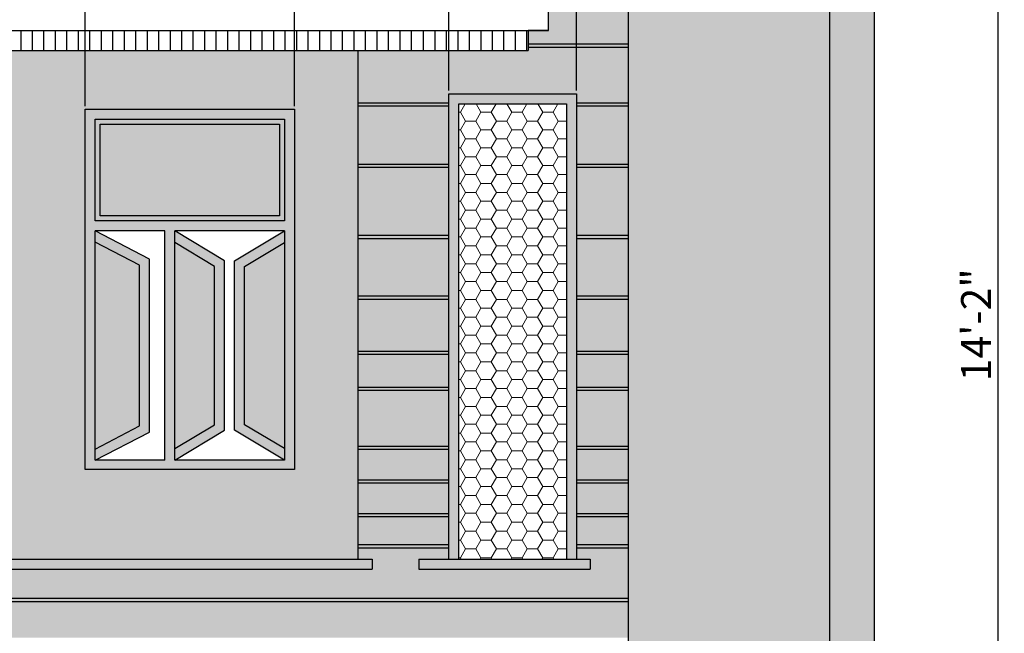
# Model space of a CAD drawing. Units: millimetres. Extents: x 4237 to 5109, y 21391 to 22486.
# Tile 3 of 17: x 4911 to 5109, y 21581 to 21704. Entities that reach past the tile are written whole.
import ezdxf

# ---------------------------------------------------------------- set-up
doc = ezdxf.new("R2010")
doc.units = ezdxf.units.MM
for name, color, linetype, lineweight in [('A-ANNO-DIMS', 2, 'Continuous', 18), ('A-ELEV', 7, 'Continuous', 25), ('A-ELEV-PATT', 252, 'Continuous', 13)]:
    doc.layers.add(name, color=color, linetype=linetype, lineweight=lineweight)
doc.styles.get("Standard").update_dxf_attribs({"font": 'arial.ttf'})
doc.dimstyles.new('ISO-25', dxfattribs={"dimtxt": 6, "dimasz": 2.5, "dimexe": 1.25, "dimexo": 0.625, "dimtad": 1, "dimdec": 1, "dimlunit": 4, "dimtxsty": 'Standard', "dimcen": 2.5, "dimadec": 0, "dimazin": 0, "dimtfac": 1, "dimtdec": 1, "dimtmove": 0, "dimatfit": 3, "dimfxl": 1, "dimarcsym": 0})

# ---------------------------------------------------------------- blocks, each defined once
blk = doc.blocks.new('*D130')
at = {"layer": 'A-ANNO-DIMS', "color": 0, "lineweight": -2, "transparency": 16777216}
for p, q in [((4878.54, 21688.54), (4878.54, 21897.84)), ((4881.04, 21896.59), (4921.78, 21896.59)), ((4924.28, 21686.68), (4924.28, 21897.84))]:
    blk.add_line(p, q, dxfattribs=at)
at = {"layer": 'A-ANNO-DIMS', "color": 0, "transparency": 16777216}
for points in [[(4881.04, 21897), (4881.04, 21896.17), (4878.54, 21896.59)], [(4921.78, 21897), (4921.78, 21896.17), (4924.28, 21896.59)]]:
    blk.add_solid(points, dxfattribs=at)
at = {"layer": 'Defpoints', "color": 0, "transparency": 16777216}
for p in [(4924.28, 21896.59), (4878.54, 21687.91), (4924.28, 21686.05)]:
    blk.add_point(p, dxfattribs=at)
at = {"layer": 'A-ANNO-DIMS', "color": 0, "transparency": 16777216, "insert": (4901.41, 21900.32), "char_height": 6, "attachment_point": 5}
blk.add_mtext('3\'-9 1/2"', dxfattribs=at)
blk = doc.blocks.new('*D131')
at = {"layer": 'A-ANNO-DIMS', "color": 0, "lineweight": -2, "transparency": 16777216}
for p, q in [((4924.28, 21686.68), (4924.28, 21897.84)), ((4926.78, 21896.59), (4963.73, 21896.59)), ((4966.23, 21686.68), (4966.23, 21897.84))]:
    blk.add_line(p, q, dxfattribs=at)
at = {"layer": 'A-ANNO-DIMS', "color": 0, "transparency": 16777216}
for points in [[(4926.78, 21897), (4926.78, 21896.17), (4924.28, 21896.59)], [(4963.73, 21897), (4963.73, 21896.17), (4966.23, 21896.59)]]:
    blk.add_solid(points, dxfattribs=at)
at = {"layer": 'Defpoints', "color": 0, "transparency": 16777216}
for p in [(4966.23, 21896.59), (4924.28, 21686.05), (4966.23, 21686.05)]:
    blk.add_point(p, dxfattribs=at)
at = {"layer": 'A-ANNO-DIMS', "color": 0, "transparency": 16777216, "insert": (4945.25, 21900.28), "char_height": 6, "attachment_point": 5}
blk.add_mtext('3\'-6"', dxfattribs=at)
blk = doc.blocks.new('*D132')
at = {"layer": 'A-ANNO-DIMS', "color": 0, "lineweight": -2, "transparency": 16777216}
for p, q in [((4966.23, 21686.68), (4966.23, 21897.84)), ((4968.73, 21896.59), (4994.7, 21896.59)), ((4997.2, 21689.78), (4997.2, 21897.84))]:
    blk.add_line(p, q, dxfattribs=at)
at = {"layer": 'A-ANNO-DIMS', "color": 0, "transparency": 16777216}
for points in [[(4968.73, 21897), (4968.73, 21896.17), (4966.23, 21896.59)], [(4994.7, 21897), (4994.7, 21896.17), (4997.2, 21896.59)]]:
    blk.add_solid(points, dxfattribs=at)
at = {"layer": 'Defpoints', "color": 0, "transparency": 16777216}
for p in [(4997.2, 21896.59), (4997.2, 21689.16), (4966.23, 21686.05)]:
    blk.add_point(p, dxfattribs=at)
at = {"layer": 'A-ANNO-DIMS', "color": 0, "transparency": 16777216, "insert": (4981.72, 21900.22), "char_height": 6, "attachment_point": 5}
blk.add_mtext('2\'-7"', dxfattribs=at)
blk = doc.blocks.new('*D133')
at = {"layer": 'A-ANNO-DIMS', "color": 0, "lineweight": -2, "transparency": 16777216}
for p, q in [((4997.2, 21689.78), (4997.2, 21897.84)), ((4999.7, 21896.59), (5020.26, 21896.59)), ((5022.76, 21689.78), (5022.76, 21897.84)), ((5022.76, 21896.59), (5056.55, 21896.59))]:
    blk.add_line(p, q, dxfattribs=at)
at = {"layer": 'A-ANNO-DIMS', "color": 0, "transparency": 16777216}
for points in [[(4999.7, 21897), (4999.7, 21896.17), (4997.2, 21896.59)], [(5020.26, 21897), (5020.26, 21896.17), (5022.76, 21896.59)]]:
    blk.add_solid(points, dxfattribs=at)
at = {"layer": 'Defpoints', "color": 0, "transparency": 16777216}
for p in [(5022.76, 21896.59), (4997.2, 21689.16), (5022.76, 21689.16)]:
    blk.add_point(p, dxfattribs=at)
at = {"layer": 'A-ANNO-DIMS', "color": 0, "transparency": 16777216, "insert": (5040.91, 21900.31), "char_height": 6, "attachment_point": 5}
blk.add_mtext('2\'-1 1/2"', dxfattribs=at)
blk = doc.blocks.new('*D134')
at = {"layer": 'A-ANNO-DIMS', "color": 0, "lineweight": -2, "transparency": 16777216}
for p, q in [((5022.76, 21689.78), (5022.76, 21897.84)), ((5025.26, 21896.59), (5080.03, 21896.59)), ((5082.53, 21809.46), (5082.53, 21897.84))]:
    blk.add_line(p, q, dxfattribs=at)
at = {"layer": 'A-ANNO-DIMS', "color": 0, "transparency": 16777216}
for points in [[(5025.26, 21897), (5025.26, 21896.17), (5022.76, 21896.59)], [(5080.03, 21897), (5080.03, 21896.17), (5082.53, 21896.59)]]:
    blk.add_solid(points, dxfattribs=at)
at = {"layer": 'Defpoints', "color": 0, "transparency": 16777216}
for p in [(5082.53, 21896.59), (5082.53, 21808.84), (5022.76, 21689.16)]:
    blk.add_point(p, dxfattribs=at)
at = {"layer": 'A-ANNO-DIMS', "color": 0, "transparency": 16777216, "insert": (5052.65, 21900.27), "char_height": 6, "attachment_point": 5}
blk.add_mtext('5\'-0"', dxfattribs=at)
blk = doc.blocks.new('*D136')
at = {"layer": 'A-ANNO-DIMS', "color": 0, "lineweight": -2, "transparency": 16777216}
for p, q in [((5074.15, 21727.84), (5108.53, 21727.84)), ((5107.28, 21560.34), (5107.28, 21725.34)), ((5083.15, 21557.84), (5108.53, 21557.84))]:
    blk.add_line(p, q, dxfattribs=at)
at = {"layer": 'A-ANNO-DIMS', "color": 0, "transparency": 16777216}
for points in [[(5106.86, 21725.34), (5107.69, 21725.34), (5107.28, 21727.84)], [(5106.86, 21560.34), (5107.69, 21560.34), (5107.28, 21557.84)]]:
    blk.add_solid(points, dxfattribs=at)
at = {"layer": 'Defpoints', "color": 0, "transparency": 16777216}
for p in [(5073.53, 21727.84), (5107.28, 21727.84), (5082.53, 21557.84)]:
    blk.add_point(p, dxfattribs=at)
at = {"layer": 'A-ANNO-DIMS', "color": 0, "transparency": 16777216, "insert": (5103.64, 21642.84), "char_height": 6, "attachment_point": 5, "rotation": 90}
blk.add_mtext('14\'-2"', dxfattribs=at)

msp = doc.modelspace()

# ---------------------------------------------------------------- hatches: boundary and pattern name
at = {"layer": 'A-ELEV-PATT'}
h = msp.add_hatch(color=256, dxfattribs=at)
h.dxf.hatch_style = 1
h.paths.add_polyline_path([(4957.45, 21796.84), (4963.45, 21796.84), (4963.45, 21727.84), (4966.45, 21727.84), (4966.45, 21796.84), (4972.45, 21796.84), (4972.45, 21727.84), (4975.45, 21727.84), (4975.45, 21796.84), (4981.45, 21796.84), (4981.45, 21727.84), (4984.45, 21727.84), (4984.45, 21796.84), (5073.53, 21796.84), (5073.53, 21557.84), (5082.53, 21557.84), (5082.53, 21808.84), (4951.45, 21808.84), (4951.45, 21727.84), (4957.45, 21727.84)])
h = msp.add_hatch(color=256, dxfattribs=at)
h.dxf.hatch_style = 1
h.paths.add_polyline_path([(5073.53, 21725.84), (5033.17, 21725.84), (5033.17, 21557.84), (5073.53, 21557.84)])
h = msp.add_hatch(color=256, dxfattribs=at)
h.dxf.hatch_style = 1
h.paths.add_polyline_path([(5033.17, 21707.76), (5017.14, 21707.76), (5017.14, 21701.84), (5013.1, 21701.84), (5013.1, 21699.14), (5033.17, 21699.14)])
h = msp.add_hatch(color=256, dxfattribs=at)
h.dxf.hatch_style = 1
h.paths.add_polyline_path([(5033.17, 21699.14), (5013.1, 21699.14), (5013.1, 21698.51), (5033.17, 21698.51)])
h = msp.add_hatch(color=256, dxfattribs=at)
h.dxf.hatch_style = 1
h.paths.add_polyline_path([(4978.93, 21697.84), (4892.07, 21697.84), (4892.07, 21623.26), (4900.89, 21623.26, -1), (4900.89, 21620.26), (4892.07, 21620.26), (4892.07, 21615.26), (4900.89, 21615.26, -1), (4900.89, 21613.26), (4892.07, 21613.26), (4892.07, 21608.26), (4900.89, 21608.26, -1), (4900.89, 21606.26), (4892.07, 21606.26), (4892.07, 21601.26), (4900.89, 21601.26, -1), (4900.89, 21599.26), (4892.07, 21599.26), (4892.07, 21595.84), (4978.93, 21595.84)])
h.paths.add_polyline_path([(4924.28, 21686.05), (4966.23, 21686.05), (4966.23, 21613.83), (4924.28, 21613.83)], flags=16)
h.paths.add_polyline_path([(4926.28, 21661.68), (4940.28, 21661.68), (4940.28, 21615.68), (4926.28, 21615.68)], flags=0)
h.paths.add_polyline_path([(4942.28, 21661.68), (4964.23, 21661.68), (4964.23, 21615.68), (4942.28, 21615.68)], flags=0)
h.paths.add_polyline_path([(4926.28, 21663.68), (4926.28, 21684.05), (4964.23, 21684.05), (4964.23, 21663.68)], flags=0)
h.paths.add_polyline_path([(4927.28, 21664.68), (4927.28, 21683.05), (4963.23, 21683.05), (4963.23, 21664.68)], flags=0)
h = msp.add_hatch(color=256, dxfattribs=at)
h.dxf.hatch_style = 1
h.paths.add_polyline_path([(5033.17, 21698.51), (5013.1, 21698.51), (5013.1, 21697.84), (4978.93, 21697.84), (4978.93, 21687.37), (4997.2, 21687.37), (4997.2, 21689.16), (5022.76, 21689.16), (5022.76, 21687.37), (5033.17, 21687.37)])
h = msp.add_hatch(color=256, dxfattribs=at)
h.dxf.hatch_style = 1
h.paths.add_polyline_path([(5022.76, 21689.16), (4997.2, 21689.16), (4997.2, 21595.84), (4999.2, 21595.84), (4999.2, 21687.16), (5020.76, 21687.16), (5020.76, 21595.84), (5022.76, 21595.84)])
h = msp.add_hatch(color=256, dxfattribs=at)
h.dxf.hatch_style = 1
h.paths.add_polyline_path([(4997.2, 21687.37), (4978.93, 21687.37), (4978.93, 21686.74), (4997.2, 21686.74)])
h = msp.add_hatch(dxfattribs=at)
h.set_pattern_fill('HONEY', color=256, scale=0.65)
h.set_pattern_definition([(0, (437.5752, 168.6426), (3.095625, 1.78725992), [2.06375, -4.1275]), (120, (437.5752, 168.6426), (-3.095625, 1.78725993), [2.06375, -4.1275]), (60, (437.5752, 168.6426), (7e-09, 3.57451985), [-4.1275, 2.06375])])
h.paths.add_polyline_path([(5020.76, 21687.16), (4999.2, 21687.16), (4999.2, 21595.84), (5020.76, 21595.84)])
h = msp.add_hatch(color=256, dxfattribs=at)
h.dxf.hatch_style = 1
h.paths.add_polyline_path([(5033.17, 21687.37), (5022.76, 21687.37), (5022.76, 21686.74), (5033.17, 21686.74)])
h = msp.add_hatch(color=256, dxfattribs=at)
h.dxf.hatch_style = 1
h.paths.add_polyline_path([(4966.23, 21686.05), (4924.28, 21686.05), (4924.28, 21613.83), (4966.23, 21613.83)])
h.paths.add_polyline_path([(4964.23, 21615.68), (4942.28, 21615.68), (4942.28, 21661.68), (4964.23, 21661.68)], flags=16)
h.paths.add_polyline_path([(4964.23, 21663.68), (4926.28, 21663.68), (4926.28, 21684.05), (4964.23, 21684.05)], flags=16)
h.paths.add_polyline_path([(4963.23, 21664.68), (4927.28, 21664.68), (4927.28, 21683.05), (4963.23, 21683.05)], flags=0)
h.paths.add_polyline_path([(4940.28, 21615.68), (4926.28, 21615.68), (4926.28, 21661.68), (4940.28, 21661.68)], flags=16)
h = msp.add_hatch(color=256, dxfattribs=at)
h.dxf.hatch_style = 1
h.paths.add_polyline_path([(4997.2, 21686.74), (4978.93, 21686.74), (4978.93, 21675.04), (4997.2, 21675.04)])
h = msp.add_hatch(color=256, dxfattribs=at)
h.dxf.hatch_style = 1
h.paths.add_polyline_path([(5033.17, 21686.74), (5022.76, 21686.74), (5022.76, 21675.04), (5033.17, 21675.04)])
h = msp.add_hatch(color=256, dxfattribs=at)
h.dxf.hatch_style = 1
h.set_gradient(color1=(122, 175, 223), color2=(215, 235, 210), name='CYLINDER')
h.paths.add_polyline_path([(4964.23, 21684.05), (4926.28, 21684.05), (4926.28, 21663.68), (4964.23, 21663.68)])
h.paths.add_polyline_path([(4963.23, 21683.05), (4963.23, 21664.68), (4927.28, 21664.68), (4927.28, 21683.05)], flags=16)
h = msp.add_hatch(color=256, dxfattribs=at)
h.dxf.hatch_style = 1
h.set_gradient(color1=(122, 175, 223), color2=(215, 235, 210), name='HEMISPHERICAL')
h.paths.add_polyline_path([(4963.23, 21683.05), (4927.28, 21683.05), (4927.28, 21664.68), (4963.23, 21664.68)])
h = msp.add_hatch(color=256, dxfattribs=at)
h.dxf.hatch_style = 1
h.paths.add_polyline_path([(4997.2, 21675.04), (4978.93, 21675.04), (4978.93, 21674.41), (4997.2, 21674.41)])
h = msp.add_hatch(color=256, dxfattribs=at)
h.dxf.hatch_style = 1
h.paths.add_polyline_path([(4997.2, 21674.41), (4978.93, 21674.41), (4978.93, 21660.8), (4997.2, 21660.8)])
h = msp.add_hatch(color=256, dxfattribs=at)
h.dxf.hatch_style = 1
h.paths.add_polyline_path([(5033.17, 21675.04), (5022.76, 21675.04), (5022.76, 21674.41), (5033.17, 21674.41)])
h = msp.add_hatch(color=256, dxfattribs=at)
h.dxf.hatch_style = 1
h.paths.add_polyline_path([(5033.17, 21674.41), (5022.76, 21674.41), (5022.76, 21660.8), (5033.17, 21660.8)])
h = msp.add_hatch(color=256, dxfattribs=at)
h.dxf.hatch_style = 1
h.paths.add_polyline_path([(4937.18, 21656.02), (4926.28, 21661.68), (4926.28, 21659.42), (4935.18, 21654.81), (4935.18, 21622.55), (4926.28, 21617.93), (4926.28, 21615.68), (4937.18, 21621.33)])
h = msp.add_hatch(color=256, dxfattribs=at)
h.dxf.hatch_style = 1
h.paths.add_polyline_path([(4952.25, 21655.67), (4942.28, 21661.68), (4942.28, 21659.34), (4950.25, 21654.54), (4950.25, 21622.81), (4942.28, 21618.01), (4942.28, 21615.68), (4952.25, 21621.68)])
h = msp.add_hatch(color=256, dxfattribs=at)
h.dxf.hatch_style = 1
h.paths.add_polyline_path([(4956.25, 21654.54), (4964.23, 21659.34), (4964.23, 21661.68), (4954.25, 21655.67), (4954.25, 21621.68), (4964.23, 21615.68), (4964.23, 21618.01), (4956.25, 21622.81)])
h = msp.add_hatch(color=256, dxfattribs=at)
h.dxf.hatch_style = 1
h.set_gradient(color1=(122, 175, 223), color2=(215, 235, 210), name='INVCYLINDER')
h.paths.add_polyline_path([(4935.18, 21654.81), (4926.28, 21659.42), (4926.28, 21617.93), (4935.18, 21622.55)])
h = msp.add_hatch(color=256, dxfattribs=at)
h.dxf.hatch_style = 1
h.paths.add_polyline_path([(4997.2, 21660.8), (4978.93, 21660.8), (4978.93, 21660.17), (4997.2, 21660.17)])
h = msp.add_hatch(color=256, dxfattribs=at)
h.dxf.hatch_style = 1
h.paths.add_polyline_path([(4997.2, 21660.17), (4978.93, 21660.17), (4978.93, 21648.61), (4997.2, 21648.61)])
h = msp.add_hatch(color=256, dxfattribs=at)
h.dxf.hatch_style = 1
h.paths.add_polyline_path([(5033.17, 21660.8), (5022.76, 21660.8), (5022.76, 21660.17), (5033.17, 21660.17)])
h = msp.add_hatch(color=256, dxfattribs=at)
h.dxf.hatch_style = 1
h.paths.add_polyline_path([(5033.17, 21660.17), (5022.76, 21660.17), (5022.76, 21648.61), (5033.17, 21648.61)])
h = msp.add_hatch(color=256, dxfattribs=at)
h.dxf.hatch_style = 1
h.set_gradient(color1=(122, 175, 223), color2=(215, 235, 210), name='INVCYLINDER')
h.paths.add_polyline_path([(4950.25, 21654.54), (4942.28, 21659.34), (4942.28, 21618.01), (4950.25, 21622.81)])
h = msp.add_hatch(color=256, dxfattribs=at)
h.dxf.hatch_style = 1
h.set_gradient(color1=(122, 175, 223), color2=(215, 235, 210), name='INVCYLINDER')
h.paths.add_polyline_path([(4964.23, 21659.34), (4956.25, 21654.54), (4956.25, 21622.81), (4964.23, 21618.01)])
h = msp.add_hatch(color=256, dxfattribs=at)
h.dxf.hatch_style = 1
h.paths.add_polyline_path([(4997.2, 21648.61), (4978.93, 21648.61), (4978.93, 21647.98), (4997.2, 21647.98)])
h = msp.add_hatch(color=256, dxfattribs=at)
h.dxf.hatch_style = 1
h.paths.add_polyline_path([(4997.2, 21647.98), (4978.93, 21647.98), (4978.93, 21637.57), (4997.2, 21637.57)])
h = msp.add_hatch(color=256, dxfattribs=at)
h.dxf.hatch_style = 1
h.paths.add_polyline_path([(5033.17, 21648.61), (5022.76, 21648.61), (5022.76, 21647.98), (5033.17, 21647.98)])
h = msp.add_hatch(color=256, dxfattribs=at)
h.dxf.hatch_style = 1
h.paths.add_polyline_path([(5033.17, 21647.98), (5022.76, 21647.98), (5022.76, 21637.57), (5033.17, 21637.57)])
h = msp.add_hatch(color=256, dxfattribs=at)
h.dxf.hatch_style = 1
h.paths.add_polyline_path([(4997.2, 21637.57), (4978.93, 21637.57), (4978.93, 21636.94), (4997.2, 21636.94)])
h = msp.add_hatch(color=256, dxfattribs=at)
h.dxf.hatch_style = 1
h.paths.add_polyline_path([(4997.2, 21636.94), (4978.93, 21636.94), (4978.93, 21630.34), (4997.2, 21630.34)])
h = msp.add_hatch(color=256, dxfattribs=at)
h.dxf.hatch_style = 1
h.paths.add_polyline_path([(5033.17, 21637.57), (5022.76, 21637.57), (5022.76, 21636.94), (5033.17, 21636.94)])
h = msp.add_hatch(color=256, dxfattribs=at)
h.dxf.hatch_style = 1
h.paths.add_polyline_path([(5033.17, 21636.94), (5022.76, 21636.94), (5022.76, 21630.34), (5033.17, 21630.34)])
h = msp.add_hatch(color=256, dxfattribs=at)
h.dxf.hatch_style = 1
h.paths.add_polyline_path([(4997.2, 21630.34), (4978.93, 21630.34), (4978.93, 21629.72), (4997.2, 21629.72)])
h = msp.add_hatch(color=256, dxfattribs=at)
h.dxf.hatch_style = 1
h.paths.add_polyline_path([(5033.17, 21630.34), (5022.76, 21630.34), (5022.76, 21629.72), (5033.17, 21629.72)])
h = msp.add_hatch(color=256, dxfattribs=at)
h.dxf.hatch_style = 1
h.paths.add_polyline_path([(4997.2, 21629.72), (4978.93, 21629.72), (4978.93, 21618.5), (4997.2, 21618.5)])
h = msp.add_hatch(color=256, dxfattribs=at)
h.dxf.hatch_style = 1
h.paths.add_polyline_path([(5033.17, 21629.72), (5022.76, 21629.72), (5022.76, 21618.5), (5033.17, 21618.5)])
h = msp.add_hatch(color=256, dxfattribs=at)
h.dxf.hatch_style = 1
h.paths.add_polyline_path([(4997.2, 21618.5), (4978.93, 21618.5), (4978.93, 21617.88), (4997.2, 21617.88)])
h = msp.add_hatch(color=256, dxfattribs=at)
h.dxf.hatch_style = 1
h.paths.add_polyline_path([(5033.17, 21618.5), (5022.76, 21618.5), (5022.76, 21617.88), (5033.17, 21617.88)])
h = msp.add_hatch(color=256, dxfattribs=at)
h.dxf.hatch_style = 1
h.paths.add_polyline_path([(4997.2, 21617.88), (4978.93, 21617.88), (4978.93, 21611.76), (4997.2, 21611.76)])
h = msp.add_hatch(color=256, dxfattribs=at)
h.dxf.hatch_style = 1
h.paths.add_polyline_path([(5033.17, 21617.88), (5022.76, 21617.88), (5022.76, 21611.76), (5033.17, 21611.76)])
h = msp.add_hatch(color=256, dxfattribs=at)
h.dxf.hatch_style = 1
h.paths.add_polyline_path([(4997.2, 21611.76), (4978.93, 21611.76), (4978.93, 21611.13), (4997.2, 21611.13)])
h = msp.add_hatch(color=256, dxfattribs=at)
h.dxf.hatch_style = 1
h.paths.add_polyline_path([(4997.2, 21611.13), (4978.93, 21611.13), (4978.93, 21605.02), (4997.2, 21605.02)])
h = msp.add_hatch(color=256, dxfattribs=at)
h.dxf.hatch_style = 1
h.paths.add_polyline_path([(5033.17, 21611.76), (5022.76, 21611.76), (5022.76, 21611.13), (5033.17, 21611.13)])
h = msp.add_hatch(color=256, dxfattribs=at)
h.dxf.hatch_style = 1
h.paths.add_polyline_path([(5033.17, 21611.13), (5022.76, 21611.13), (5022.76, 21605.02), (5033.17, 21605.02)])
h = msp.add_hatch(color=256, dxfattribs=at)
h.dxf.hatch_style = 1
h.paths.add_polyline_path([(4997.2, 21605.02), (4978.93, 21605.02), (4978.93, 21604.39), (4997.2, 21604.39)])
h = msp.add_hatch(color=256, dxfattribs=at)
h.dxf.hatch_style = 1
h.paths.add_polyline_path([(4997.2, 21604.39), (4978.93, 21604.39), (4978.93, 21598.78), (4997.2, 21598.78)])
h = msp.add_hatch(color=256, dxfattribs=at)
h.dxf.hatch_style = 1
h.paths.add_polyline_path([(5033.17, 21605.02), (5022.76, 21605.02), (5022.76, 21604.39), (5033.17, 21604.39)])
h = msp.add_hatch(color=256, dxfattribs=at)
h.dxf.hatch_style = 1
h.paths.add_polyline_path([(5033.17, 21604.39), (5022.76, 21604.39), (5022.76, 21598.78), (5033.17, 21598.78)])
h = msp.add_hatch(color=256, dxfattribs=at)
h.dxf.hatch_style = 1
h.paths.add_polyline_path([(4997.2, 21598.78), (4978.93, 21598.78), (4978.93, 21598.15), (4997.2, 21598.15)])
h = msp.add_hatch(color=256, dxfattribs=at)
h.dxf.hatch_style = 1
h.paths.add_polyline_path([(5033.17, 21598.78), (5022.76, 21598.78), (5022.76, 21598.15), (5033.17, 21598.15)])
h = msp.add_hatch(color=256, dxfattribs=at)
h.dxf.hatch_style = 1
h.paths.add_polyline_path([(5033.17, 21598.15), (5022.76, 21598.15), (5022.76, 21595.84), (5025.55, 21595.84), (5025.55, 21593.84), (4991.17, 21593.84), (4991.17, 21595.84), (4997.2, 21595.84), (4997.2, 21598.15), (4978.93, 21598.15), (4978.93, 21595.84), (4981.84, 21595.84), (4981.84, 21593.84), (4793.12, 21593.84), (4793.12, 21588.01), (5033.17, 21588.01)])
h = msp.add_hatch(color=256, dxfattribs=at)
h.dxf.hatch_style = 1
h.paths.add_polyline_path([(4981.84, 21595.84), (4793.12, 21595.84), (4793.12, 21593.84), (4981.84, 21593.84)])
h = msp.add_hatch(color=256, dxfattribs=at)
h.dxf.hatch_style = 1
h.paths.add_polyline_path([(5025.55, 21595.84), (4991.17, 21595.84), (4991.17, 21593.84), (5025.55, 21593.84)])
h = msp.add_hatch(color=256, dxfattribs=at)
h.dxf.hatch_style = 1
h.paths.add_polyline_path([(5033.17, 21588.01), (4793.12, 21588.01), (4793.12, 21587.38), (5033.17, 21587.38)])
h = msp.add_hatch(color=256, dxfattribs=at)
h.dxf.hatch_style = 1
h.paths.add_polyline_path([(5033.17, 21587.38), (4793.12, 21587.38), (4793.12, 21581.84), (4834.56, 21581.84), (4834.56, 21580.12), (5033.17, 21580.12)])

# ---------------------------------------------------------------- linework, layer by layer
at = {"layer": 'A-ELEV'}
for p, q in [((5082.53, 21425.84), (5082.53, 21808.84)), ((5073.53, 21425.84), (5073.53, 21796.84)), ((5033.17, 21557.84), (5033.17, 21772.84)), ((5017.14, 21701.84), (5017.14, 21727.84)), ((4757.12, 21701.84), (5017.14, 21701.84)), ((4911.38, 21701.84), (4911.38, 21697.84)), ((4913.68, 21701.84), (4913.68, 21697.84)), ((4915.98, 21701.84), (4915.98, 21697.84)), ((4918.28, 21701.84), (4918.28, 21697.84)), ((4920.59, 21701.84), (4920.59, 21697.84)), ((4922.89, 21701.84), (4922.89, 21697.84)), ((4925.19, 21701.84), (4925.19, 21697.84)), ((4927.49, 21701.84), (4927.49, 21697.84)), ((4929.8, 21701.84), (4929.8, 21697.84)), ((4932.1, 21701.84), (4932.1, 21697.84)), ((4934.4, 21701.84), (4934.4, 21697.84)), ((4936.7, 21701.84), (4936.7, 21697.84)), ((4939.01, 21701.84), (4939.01, 21697.84)), ((4941.31, 21701.84), (4941.31, 21697.84)), ((4943.61, 21701.84), (4943.61, 21697.84)), ((4945.91, 21701.84), (4945.91, 21697.84)), ((4948.22, 21701.84), (4948.22, 21697.84)), ((4950.52, 21701.84), (4950.52, 21697.84)), ((4952.82, 21701.84), (4952.82, 21697.84)), ((4955.12, 21701.84), (4955.12, 21697.84)), ((4957.42, 21701.84), (4957.42, 21697.84)), ((4959.73, 21701.84), (4959.73, 21697.84)), ((4962.03, 21701.84), (4962.03, 21697.84)), ((4964.33, 21701.84), (4964.33, 21697.84)), ((4966.63, 21701.84), (4966.63, 21697.84)), ((4968.94, 21701.84), (4968.94, 21697.84)), ((4971.24, 21701.84), (4971.24, 21697.84)), ((4973.54, 21701.84), (4973.54, 21697.84)), ((4975.84, 21701.84), (4975.84, 21697.84)), ((4978.15, 21701.84), (4978.15, 21697.84)), ((4980.45, 21701.84), (4980.45, 21697.84)), ((4982.75, 21701.84), (4982.75, 21697.84)), ((4985.05, 21701.84), (4985.05, 21697.84)), ((4987.36, 21701.84), (4987.36, 21697.84)), ((4989.66, 21701.84), (4989.66, 21697.84)), ((4992.06, 21701.84), (4992.06, 21697.84)), ((4994.37, 21701.84), (4994.37, 21697.84)), ((4996.67, 21701.84), (4996.67, 21697.84)), ((4998.97, 21701.84), (4998.97, 21697.84)), ((5001.27, 21701.84), (5001.27, 21697.84)), ((5003.58, 21701.84), (5003.58, 21697.84)), ((5005.88, 21701.84), (5005.88, 21697.84)), ((5008.18, 21701.84), (5008.18, 21697.84)), ((5010.48, 21701.84), (5010.48, 21697.84)), ((5012.78, 21701.84), (5012.78, 21697.84)), ((5017.14, 21701.84), (5013.1, 21701.84)), ((5013.1, 21701.84), (5013.1, 21697.84)), ((5013.1, 21699.14), (5033.17, 21699.14)), ((4757.12, 21697.84), (5013.1, 21697.84)), ((4978.93, 21697.84), (4978.93, 21595.84)), ((5013.1, 21698.51), (5033.17, 21698.51)), ((4978.93, 21687.37), (4997.2, 21687.37)), ((5022.76, 21687.37), (5033.17, 21687.37)), ((4978.93, 21686.74), (4997.2, 21686.74)), ((5022.76, 21686.74), (5033.17, 21686.74)), ((4978.93, 21675.04), (4997.2, 21675.04)), ((4978.93, 21674.41), (4997.2, 21674.41)), ((5022.76, 21675.04), (5033.17, 21675.04)), ((5022.76, 21674.41), (5033.17, 21674.41)), ((4940.28, 21661.68), (4926.28, 21661.68)), ((4926.28, 21615.68), (4926.28, 21661.68)), ((4940.28, 21615.68), (4940.28, 21661.68)), ((4964.23, 21661.68), (4942.28, 21661.68)), ((4942.28, 21615.68), (4942.28, 21661.68)), ((4964.23, 21661.68), (4964.23, 21615.68)), ((4978.93, 21660.8), (4997.2, 21660.8)), ((4978.93, 21660.17), (4997.2, 21660.17)), ((5022.76, 21660.8), (5033.17, 21660.8)), ((5022.76, 21660.17), (5033.17, 21660.17)), ((4978.93, 21648.61), (4997.2, 21648.61)), ((4978.93, 21647.98), (4997.2, 21647.98)), ((5022.76, 21648.61), (5033.17, 21648.61)), ((5022.76, 21647.98), (5033.17, 21647.98)), ((4978.93, 21637.57), (4997.2, 21637.57)), ((4978.93, 21636.94), (4997.2, 21636.94)), ((5022.76, 21637.57), (5033.17, 21637.57)), ((5022.76, 21636.94), (5033.17, 21636.94)), ((4978.93, 21630.34), (4997.2, 21630.34)), ((5022.76, 21630.34), (5033.17, 21630.34)), ((4978.93, 21629.72), (4997.2, 21629.72)), ((5022.76, 21629.72), (5033.17, 21629.72)), ((4978.93, 21618.5), (4997.2, 21618.5)), ((5022.76, 21618.5), (5033.17, 21618.5)), ((4978.93, 21617.88), (4997.2, 21617.88)), ((5022.76, 21617.88), (5033.17, 21617.88)), ((4940.28, 21615.68), (4926.28, 21615.68)), ((4964.23, 21615.68), (4942.28, 21615.68)), ((4978.93, 21611.76), (4997.2, 21611.76)), ((4978.93, 21611.13), (4997.2, 21611.13)), ((5022.76, 21611.76), (5033.17, 21611.76)), ((5022.76, 21611.13), (5033.17, 21611.13)), ((4978.93, 21605.02), (4997.2, 21605.02)), ((4978.93, 21604.39), (4997.2, 21604.39)), ((5022.76, 21605.02), (5033.17, 21605.02)), ((5022.76, 21604.39), (5033.17, 21604.39)), ((4978.93, 21598.78), (4997.2, 21598.78)), ((5022.76, 21598.78), (5033.17, 21598.78)), ((4978.93, 21598.15), (4997.2, 21598.15)), ((5022.76, 21598.15), (5033.17, 21598.15)), ((4793.12, 21595.84), (4981.84, 21595.84)), ((4981.84, 21595.84), (4981.84, 21593.84)), ((4991.17, 21595.84), (5025.55, 21595.84)), ((4991.17, 21595.84), (4991.17, 21593.84)), ((5025.55, 21595.84), (5025.55, 21593.84)), ((4793.12, 21593.84), (4981.84, 21593.84)), ((4991.17, 21593.84), (5025.55, 21593.84)), ((4793.12, 21588.01), (5033.17, 21588.01)), ((4793.12, 21587.38), (5033.17, 21587.38))]:
    msp.add_line(p, q, dxfattribs=at)
for points in [[(4997.2, 21595.84), (4997.2, 21689.16), (5022.76, 21689.16), (5022.76, 21595.84)], [(4999.2, 21595.84), (4999.2, 21687.16), (5020.76, 21687.16), (5020.76, 21595.84)], [(4926.28, 21615.68), (4937.18, 21621.33), (4937.18, 21656.02), (4926.28, 21661.68)], [(4942.28, 21615.68), (4952.25, 21621.68), (4952.25, 21655.67), (4942.28, 21661.68)], [(4964.23, 21615.68), (4954.25, 21621.68), (4954.25, 21655.67), (4964.23, 21661.68)], [(4926.28, 21617.93), (4935.18, 21622.55), (4935.18, 21654.81), (4926.28, 21659.42)], [(4942.28, 21618.01), (4950.25, 21622.81), (4950.25, 21654.54), (4942.28, 21659.34)], [(4964.23, 21618.01), (4956.25, 21622.81), (4956.25, 21654.54), (4964.23, 21659.34)]]:
    msp.add_lwpolyline(points, dxfattribs=at)
for points in [[(4924.28, 21686.05), (4966.23, 21686.05), (4966.23, 21613.83), (4924.28, 21613.83)], [(4964.23, 21684.05), (4964.23, 21663.68), (4926.28, 21663.68), (4926.28, 21684.05)], [(4963.23, 21683.05), (4963.23, 21664.68), (4927.28, 21664.68), (4927.28, 21683.05)]]:
    msp.add_lwpolyline(points, close=True, dxfattribs=at)

# ---------------------------------------------------------------- dimensions: what is measured, and where the dimension line sits
at = {"layer": 'A-ANNO-DIMS'}
for base, p1, p2, picture, middle in [((4924.28, 21896.59), (4878.54, 21687.91), (4924.28, 21686.05), '*D130', (4901.41, 21900.32)), ((5022.76, 21896.59), (4997.2, 21689.16), (5022.76, 21689.16), '*D133', (5040.91, 21900.31)), ((4966.2267, 21896.586), (4924.2801, 21686.0515), (4966.2267, 21686.0515), '*D131', (4945.2534, 21900.2765)), ((4997.2, 21896.59), (4966.23, 21686.05), (4997.2, 21689.16), '*D132', (4981.72, 21900.22)), ((5082.53, 21896.59), (5022.76, 21689.16), (5082.53, 21808.84), '*D134', (5052.65, 21900.27))]:
    dim = msp.add_linear_dim(base=base, p1=p1, p2=p2, dimstyle='ISO-25', override={"dimdec": 1, "dimlfac": 1, "dimrnd": 0, "dimzin": 1, "dimdsep": 46, "dimlunit": 4, "dimfrac": 2}, dxfattribs=at)
    dim.commit()
    dim.dimension.update_dxf_attribs({"geometry": picture, "text_midpoint": middle})
dim = msp.add_linear_dim(base=(5107.28, 21727.84), p1=(5082.53, 21557.84), p2=(5073.53, 21727.84), angle=90, dimstyle='ISO-25', override={"dimdec": 1, "dimlfac": 1, "dimrnd": 0, "dimzin": 1, "dimdsep": 46, "dimlunit": 4, "dimfrac": 2}, dxfattribs=at)
dim.commit()
dim.dimension.update_dxf_attribs({"geometry": '*D136', "text_midpoint": (5103.64, 21642.84)})

doc.saveas('drawing.dxf')
